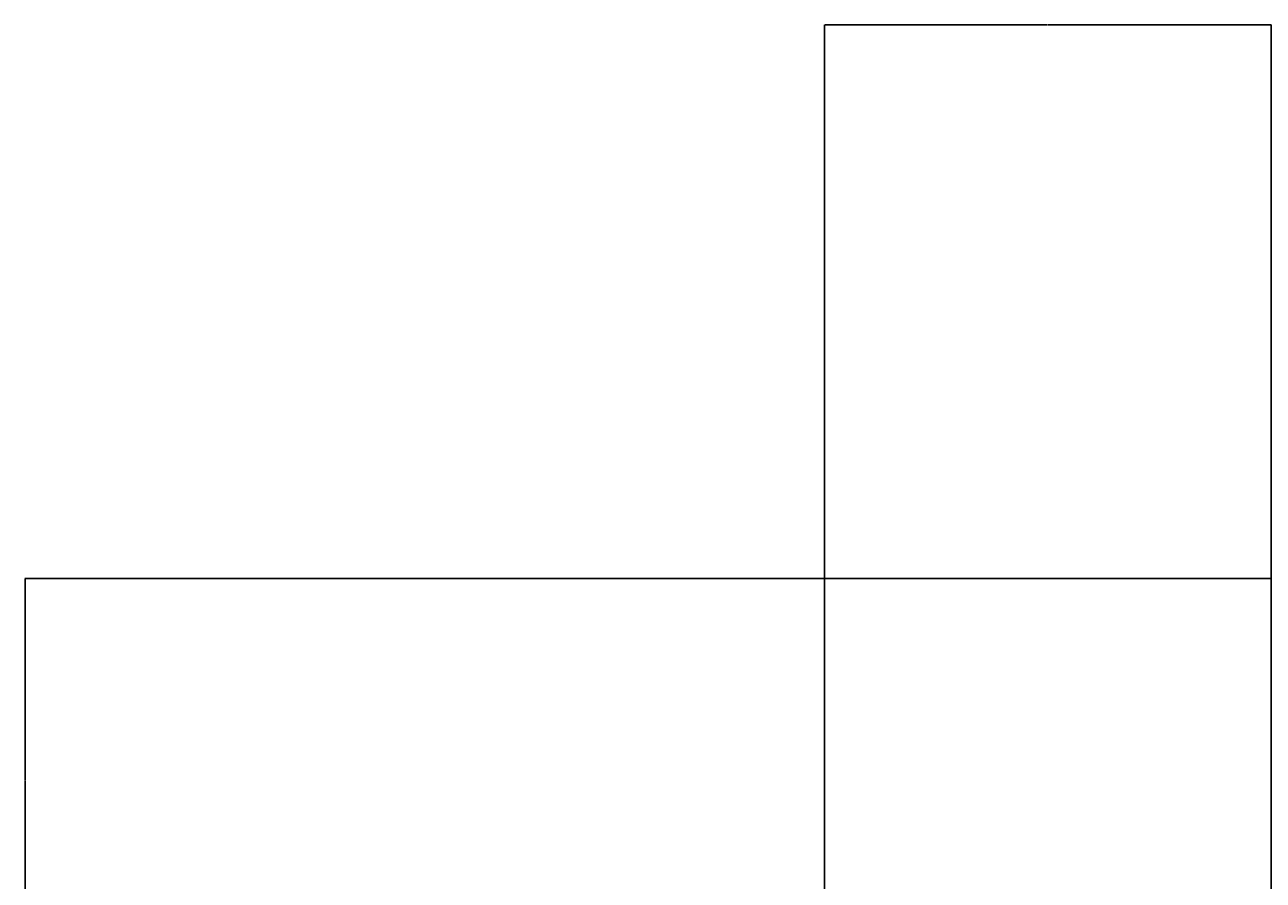
# Model space of a CAD drawing. Units: inches. Extents: x -69 to 2453, y 4803 to 7122.
# Tile 4 of 9: x -69 to 1203, y 6243 to 7122. Entities that reach past the tile are written whole.
import ezdxf

# ---------------------------------------------------------------- set-up
doc = ezdxf.new("R2010")
doc.units = ezdxf.units.IN
doc.layers.add('A-ANNO-DIMS', color=2, linetype='Continuous', lineweight=18)
doc.styles.get("Standard").update_dxf_attribs({"font": 'arial.ttf'})
doc.dimstyles.get("Standard").update_dxf_attribs({"dimtxt": 0.18, "dimasz": 0.18, "dimexe": 0.18, "dimexo": 0.0625, "dimgap": 0.09, "dimtad": 0, "dimtih": 1, "dimtoh": 1, "dimdec": 4, "dimzin": 0, "dimdsep": 46, "dimtxsty": 'Standard', "dimcen": 0.09, "dimadec": 0, "dimazin": 0, "dimtfac": 1, "dimtdec": 4, "dimtofl": 0, "dimtmove": 0, "dimatfit": 3, "dimfxl": 1, "dimtolj": 1, "dimtzin": 0, "dimarcsym": 0})

# ---------------------------------------------------------------- blocks, each defined once
blk = doc.blocks.new('*D100')
at = {"layer": 'A-ANNO-DIMS', "color": 0, "lineweight": -2, "transparency": 16777216}
for p, q in [((752.5, 6159.8), (752.5, 7121.6)), ((752.7, 7121.5), (981.7, 7121.5)), ((1211.3, 7121.5), (982.3, 7121.5)), ((1211.5, 6159.8), (1211.5, 7121.6))]:
    blk.add_line(p, q, dxfattribs=at)
at = {"layer": 'A-ANNO-DIMS', "color": 0, "transparency": 16777216}
for points in [[(752.7, 7121.5), (752.7, 7121.4), (752.5, 7121.5)], [(1211.3, 7121.5), (1211.3, 7121.4), (1211.5, 7121.5)]]:
    blk.add_solid(points, dxfattribs=at)
at = {"layer": 'Defpoints', "color": 0, "transparency": 16777216}
for p in [(1211.5, 7121.5), (752.5, 6159.7), (1211.5, 6159.7)]:
    blk.add_point(p, dxfattribs=at)
at = {"layer": 'A-ANNO-DIMS', "color": 0, "transparency": 16777216, "insert": (982, 7121.5), "char_height": 0.18, "attachment_point": 5}
blk.add_mtext('\\A1;459', dxfattribs=at)
blk = doc.blocks.new('*D103')
at = {"layer": 'A-ANNO-DIMS', "color": 0, "lineweight": -2, "transparency": 16777216}
for p, q in [((1241.4, 6552.7), (-69.4, 6552.7)), ((-69.2, 6552.5), (-69.2, 6345.9)), ((-69.2, 6138.9), (-69.2, 6345.5)), ((1241.4, 6138.7), (-69.4, 6138.7))]:
    blk.add_line(p, q, dxfattribs=at)
at = {"layer": 'A-ANNO-DIMS', "color": 0, "transparency": 16777216}
for points in [[(-69.3, 6552.5), (-69.2, 6552.5), (-69.2, 6552.7)], [(-69.3, 6138.9), (-69.2, 6138.9), (-69.2, 6138.7)]]:
    blk.add_solid(points, dxfattribs=at)
at = {"layer": 'Defpoints', "color": 0, "transparency": 16777216}
for p in [(-69.2, 6552.7), (1241.5, 6552.7), (1241.5, 6138.7)]:
    blk.add_point(p, dxfattribs=at)
at = {"layer": 'A-ANNO-DIMS', "color": 0, "transparency": 16777216, "insert": (-69.2, 6345.7), "char_height": 0.18, "attachment_point": 5}
blk.add_mtext('\\A1;414', dxfattribs=at)

msp = doc.modelspace()

# ---------------------------------------------------------------- dimensions: what is measured, and where the dimension line sits
at = {"layer": 'A-ANNO-DIMS'}
dim = msp.add_linear_dim(base=(1211.5, 7121.5), p1=(752.5, 6159.7), p2=(1211.5, 6159.7), dimstyle='Standard', override={"dimdec": 0, "dimlfac": 1, "dimrnd": 0, "dimzin": 0, "dimdsep": 46, "dimlunit": 2}, dxfattribs=at)
dim.commit()
dim.dimension.update_dxf_attribs({"geometry": '*D100', "text_midpoint": (982, 7121.5)})
dim = msp.add_linear_dim(base=(-69.2, 6552.7), p1=(1241.5, 6138.7), p2=(1241.5, 6552.7), angle=90, dimstyle='Standard', override={"dimdec": 0, "dimlfac": 1, "dimrnd": 0, "dimzin": 0, "dimdsep": 46, "dimlunit": 2}, dxfattribs=at)
dim.commit()
dim.dimension.update_dxf_attribs({"geometry": '*D103', "text_midpoint": (-69.2, 6345.7)})

doc.saveas('drawing.dxf')
